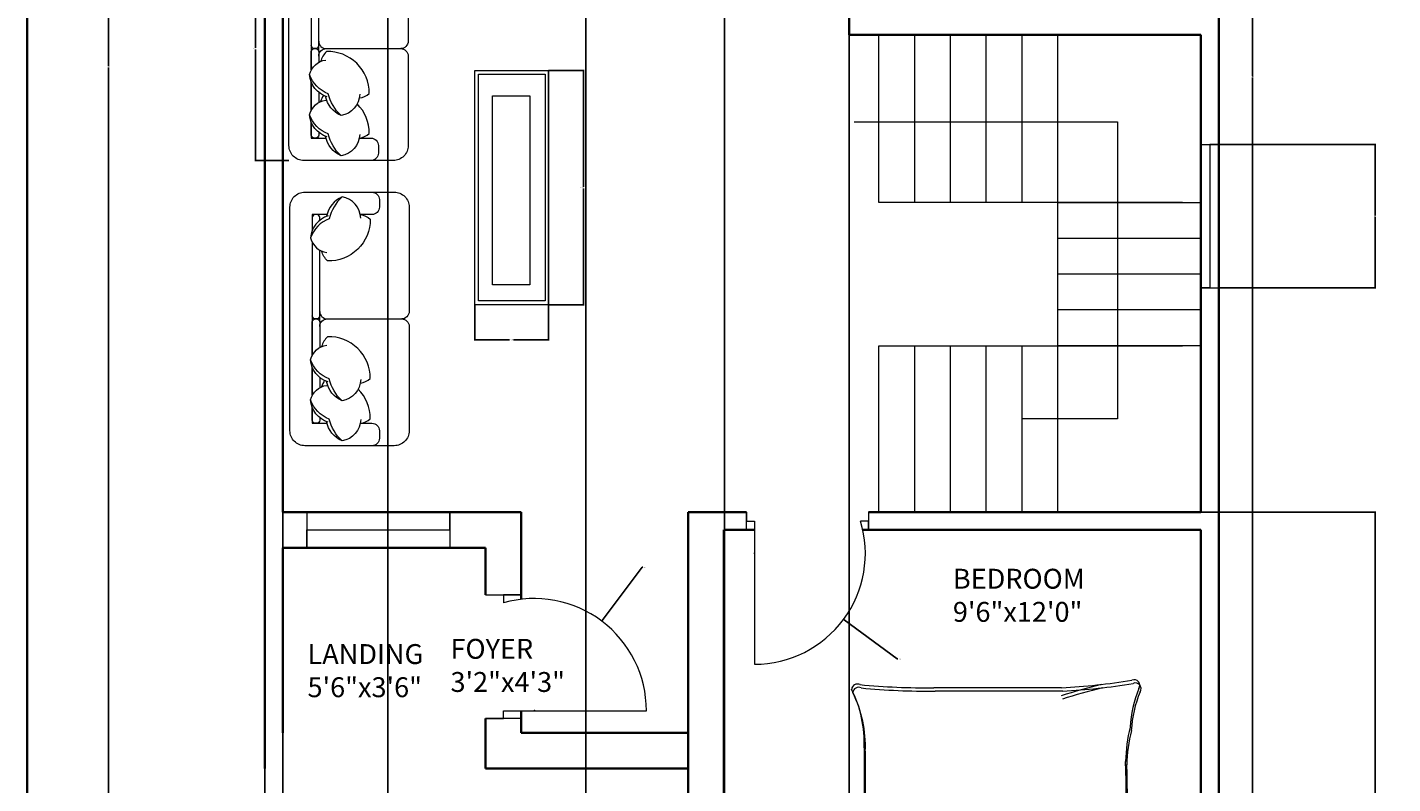
# Model space of a CAD drawing. Units: inches. Extents: x 1734 to 2405, y 1500 to 2491.
# Tile 7 of 14: x 1734 to 2078, y 1888 to 2078. Entities that reach past the tile are written whole.
import ezdxf

# ---------------------------------------------------------------- set-up
doc = ezdxf.new("R2010")
doc.units = ezdxf.units.IN
for name, color, linetype, lineweight in [('A-ANNO-DIMS', 2, 'Continuous', 18), ('A-ANNO-TTLB', 7, 'Continuous', 35), ('A-AREA-IDEN', 7, 'Continuous', 18), ('A-DOOR', 3, 'Continuous', 18), ('A-FLOR-STRS', 7, 'Continuous', 18), ('A-FURN', 8, 'Continuous', 13), ('A-GLAZ', 4, 'Continuous', 18), ('A-WALL', 7, 'Continuous', 35), ('C-PROP', 7, 'Continuous', 25)]:
    doc.layers.add(name, color=color, linetype=linetype, lineweight=lineweight)
doc.styles.get("Standard").update_dxf_attribs({"font": 'arial.ttf'})
doc.dimstyles.get("Standard").update_dxf_attribs({"dimtxt": 0.18, "dimasz": 0.18, "dimexe": 0.18, "dimexo": 0.0625, "dimgap": 0.09, "dimtad": 0, "dimtih": 1, "dimtoh": 1, "dimdec": 4, "dimzin": 0, "dimdsep": 46, "dimtxsty": 'Standard', "dimcen": 0.09, "dimadec": 0, "dimazin": 0, "dimtfac": 1, "dimtdec": 4, "dimtofl": 0, "dimtmove": 0, "dimatfit": 3, "dimfxl": 1, "dimtolj": 1, "dimtzin": 0, "dimarcsym": 0})

# ---------------------------------------------------------------- blocks, each defined once
blk = doc.blocks.new('BED-DOUBLE')
for p, q in [((81.88, 67.96), (105.53, 67.96)), ((81.88, 67.96), (105.53, 67.96)), ((82.71, 68.26), (106.37, 68.26)), ((82.71, 68.26), (106.37, 68.26)), ((83.83, 60.38), (82.88, 67.03)), ((82.88, 67.03), (87.04, 66.28)), ((83.83, 60.38), (82.88, 67.03)), ((82.88, 67.03), (87.04, 66.28)), ((84.66, 60.68), (83.72, 67.33)), ((83.72, 67.33), (87.87, 66.58)), ((84.66, 60.68), (83.72, 67.33)), ((83.72, 67.33), (87.87, 66.58)), ((87.04, 66.28), (89.12, 66.66)), ((87.04, 66.28), (89.12, 66.66)), ((87.87, 66.58), (89.95, 66.95)), ((87.87, 66.58), (89.95, 66.95)), ((89.12, 66.66), (93.84, 65.9)), ((89.12, 66.66), (93.84, 65.9)), ((89.95, 66.95), (94.67, 66.2)), ((89.95, 66.95), (94.67, 66.2)), ((93.65, 67.22), (92.33, 66.47)), ((93.65, 67.22), (92.33, 66.47)), ((94.48, 67.52), (93.16, 66.77)), ((94.48, 67.52), (93.16, 66.77)), ((97.05, 66.66), (93.65, 67.22)), ((97.05, 66.66), (93.65, 67.22)), ((93.84, 65.9), (97.42, 64.58)), ((93.84, 65.9), (97.42, 64.58)), ((97.88, 66.95), (94.48, 67.52)), ((97.88, 66.95), (94.48, 67.52)), ((94.67, 66.2), (98.26, 64.88)), ((94.67, 66.2), (98.26, 64.88)), ((101.2, 67.41), (97.05, 66.66)), ((101.2, 67.41), (97.05, 66.66)), ((102.04, 67.71), (97.88, 66.95)), ((102.04, 67.71), (97.88, 66.95)), ((101.17, 67.41), (101.6, 61.81)), ((101.17, 67.41), (101.6, 61.82)), ((102.01, 67.7), (102.44, 62.11)), ((102.01, 67.7), (102.44, 62.11)), ((103.53, 67.96), (103.53, 5.54)), ((103.53, 67.96), (103.53, 5.54)), ((104.36, 68.26), (104.36, 5.84)), ((104.36, 68.26), (104.36, 5.84)), ((106.37, 5.54), (106.37, 67.96)), ((85.12, 64.16), (84.25, 58.9)), ((85.12, 64.16), (84.25, 58.9)), ((85.96, 64.46), (85.09, 59.2)), ((85.96, 64.46), (85.09, 59.2)), ((102.41, 61.98), (102.04, 56.98)), ((102.41, 61.98), (102.04, 56.98)), ((102.44, 62.11), (102.41, 61.98)), ((102.44, 62.11), (102.41, 61.98)), ((84.25, 58.9), (83.69, 49.74)), ((84.25, 58.9), (83.69, 49.74)), ((84.25, 58.9), (83.83, 60.38)), ((84.25, 58.9), (83.83, 60.38)), ((85.09, 59.2), (84.52, 50.04)), ((85.09, 59.2), (84.52, 50.04)), ((85.09, 59.2), (84.66, 60.68)), ((85.09, 59.2), (84.66, 60.68)), ((101.58, 61.68), (101.2, 56.68)), ((101.58, 61.68), (101.2, 56.68)), ((101.6, 61.82), (101.58, 61.68)), ((101.6, 61.81), (101.58, 61.68)), ((101.2, 56.68), (99.88, 49.51)), ((101.2, 56.68), (99.88, 49.51)), ((102.04, 56.98), (100.71, 49.81)), ((102.04, 56.98), (100.71, 49.81)), ((2.04, 52.82), (2.04, 20.68)), ((2.04, 52.82), (2.04, 20.68)), ((2.87, 53.12), (2.87, 20.98)), ((2.87, 53.12), (2.87, 20.98)), ((100.64, 53.1), (101.58, 50.45)), ((100.64, 53.1), (101.58, 50.45)), ((101.47, 53.4), (102.41, 50.75)), ((101.47, 53.39), (102.41, 50.75)), ((83.69, 49.74), (84.42, 47.18)), ((83.69, 49.74), (84.42, 47.18)), ((84.52, 50.04), (85.25, 47.48)), ((84.52, 50.04), (85.25, 47.48)), ((101.58, 50.45), (102.52, 46.68)), ((101.58, 50.45), (102.52, 46.68)), ((102.41, 50.75), (103.36, 46.98)), ((102.41, 50.75), (103.36, 46.98)), ((84.42, 47.18), (83.89, 40.48)), ((84.42, 47.18), (83.89, 40.48)), ((84.29, 41.02), (85.72, 45.13)), ((84.29, 41.02), (85.72, 45.12)), ((85.25, 47.48), (84.72, 40.78)), ((85.25, 47.48), (84.72, 40.78)), ((85.13, 41.32), (86.55, 45.42)), ((85.13, 41.32), (86.55, 45.42)), ((102.52, 46.26), (102.33, 40.45)), ((102.52, 46.26), (102.33, 40.45)), ((102.52, 46.68), (102.52, 46.26)), ((102.52, 46.68), (102.52, 46.26)), ((103.36, 46.56), (103.17, 40.75)), ((103.36, 46.56), (103.17, 40.75)), ((103.36, 46.98), (103.36, 46.56)), ((103.36, 46.98), (103.36, 46.56)), ((85.13, 38.11), (85.13, 41.32)), ((85.13, 38.11), (85.13, 41.32)), ((84.29, 37.81), (84.29, 41.02)), ((84.29, 37.81), (84.29, 41.02)), ((87.79, 37.81), (84.29, 37.81)), ((87.79, 37.81), (84.29, 37.81)), ((88.63, 38.11), (85.13, 38.11)), ((88.63, 38.11), (85.13, 38.11)), ((90.25, 37.05), (87.79, 37.81)), ((90.25, 37.05), (87.79, 37.81)), ((91.08, 37.35), (88.63, 38.11)), ((91.08, 37.35), (88.63, 38.11)), ((96.1, 37.81), (91.95, 37.05)), ((96.1, 37.81), (91.95, 37.05)), ((96.94, 38.11), (92.78, 37.35)), ((96.94, 38.11), (92.78, 37.35)), ((103.09, 38.56), (96.1, 37.81)), ((103.09, 38.56), (96.1, 37.81)), ((103.92, 38.86), (96.94, 38.11)), ((103.92, 38.86), (96.94, 38.11)), ((102.33, 40.45), (103.09, 38.56)), ((102.33, 40.45), (103.09, 38.56)), ((103.17, 40.75), (103.92, 38.86)), ((103.17, 40.75), (103.92, 38.86)), ((86.97, 35.76), (83.47, 35.54)), ((86.97, 35.76), (83.47, 35.54)), ((83.47, 35.54), (83.67, 32.34)), ((83.47, 35.54), (83.67, 32.34)), ((87.8, 36.06), (84.3, 35.84)), ((87.8, 36.06), (84.3, 35.84)), ((84.3, 35.84), (84.51, 32.63)), ((84.3, 35.84), (84.51, 32.64)), ((89.37, 36.67), (86.97, 35.76)), ((89.37, 36.67), (86.97, 35.76)), ((90.2, 36.96), (87.8, 36.06)), ((90.2, 36.96), (87.8, 36.06)), ((91.06, 36.77), (89.37, 36.67)), ((91.06, 36.77), (89.37, 36.67)), ((91.9, 37.07), (90.2, 36.96)), ((91.9, 37.07), (90.2, 36.96)), ((91.95, 37.05), (90.25, 37.05)), ((91.95, 37.05), (90.25, 37.05)), ((95.26, 36.28), (91.06, 36.77)), ((95.26, 36.28), (91.06, 36.77)), ((92.78, 37.35), (91.08, 37.35)), ((92.78, 37.35), (91.08, 37.35)), ((96.09, 36.57), (91.9, 37.07)), ((96.09, 36.58), (91.9, 37.07)), ((102.28, 35.96), (95.26, 36.28)), ((102.28, 35.96), (95.26, 36.28)), ((103.11, 36.26), (96.09, 36.58)), ((103.11, 36.26), (96.09, 36.57)), ((101.64, 34.03), (102.28, 35.96)), ((101.64, 34.03), (102.28, 35.96)), ((102.48, 34.33), (103.11, 36.26)), ((102.48, 34.33), (103.11, 36.26)), ((82.83, 32.98), (74.35, 27.51)), ((82.83, 32.98), (74.35, 27.51)), ((83.66, 33.28), (75.18, 27.8)), ((83.66, 33.28), (75.18, 27.8)), ((83.67, 32.34), (85.35, 28.33)), ((83.67, 32.34), (85.35, 28.33)), ((84.51, 32.64), (86.18, 28.63)), ((84.51, 32.63), (86.18, 28.62)), ((102.19, 28.24), (101.64, 34.03)), ((102.19, 28.24), (101.64, 34.03)), ((103.03, 28.54), (102.48, 34.33)), ((103.03, 28.54), (102.48, 34.33)), ((74.35, 27.51), (68.49, 25.28)), ((74.35, 27.51), (68.49, 25.28)), ((75.18, 27.8), (69.32, 25.58)), ((75.18, 27.8), (69.32, 25.58)), ((79, 19.42), (82.83, 30.31)), ((79, 19.41), (82.83, 30.3)), ((79.83, 19.71), (83.66, 30.6)), ((79.83, 19.71), (83.66, 30.6)), ((85.12, 29.97), (84.25, 24.7)), ((85.12, 29.97), (84.25, 24.7)), ((85.96, 30.27), (85.09, 25)), ((85.96, 30.27), (85.09, 25)), ((101.51, 24), (102.22, 27.83)), ((101.51, 24), (102.22, 27.83)), ((102.22, 27.83), (102.19, 28.24)), ((102.22, 27.83), (102.19, 28.24)), ((102.35, 24.3), (103.05, 28.12)), ((102.35, 24.3), (103.05, 28.12)), ((103.05, 28.12), (103.03, 28.54)), ((103.05, 28.12), (103.03, 28.54)), ((68.49, 25.28), (65.86, 24.88)), ((68.49, 25.28), (65.86, 24.88)), ((65.86, 24.88), (66.67, 21.64)), ((65.86, 24.88), (66.67, 21.64)), ((69.32, 25.58), (66.69, 25.17)), ((69.32, 25.58), (66.69, 25.17)), ((66.69, 25.17), (67.5, 21.94)), ((66.69, 25.17), (67.5, 21.94)), ((84.25, 24.7), (83.69, 15.55)), ((84.25, 24.7), (83.69, 15.55)), ((85.09, 25), (84.52, 15.84)), ((85.09, 25), (84.52, 15.85)), ((101.52, 17.76), (99.76, 24.83)), ((101.52, 17.76), (99.76, 24.83)), ((102.36, 18.05), (100.59, 25.13)), ((102.36, 18.05), (100.59, 25.13)), ((101.57, 21.6), (102.35, 24.3)), ((101.57, 21.6), (102.35, 24.3)), ((66.67, 21.64), (67.88, 19.01)), ((66.67, 21.64), (67.88, 19.01)), ((67.5, 21.94), (68.72, 19.31)), ((67.5, 21.94), (68.72, 19.31)), ((100.73, 21.3), (101.51, 24)), ((100.73, 21.3), (101.51, 24)), ((67.88, 19.01), (68.49, 14.56)), ((67.88, 19.01), (68.49, 14.56)), ((68.72, 19.31), (69.32, 14.86)), ((68.72, 19.31), (69.32, 14.86)), ((76.37, 12.13), (79, 19.42)), ((76.37, 12.13), (79, 19.41)), ((77.21, 12.43), (79.83, 19.71)), ((77.21, 12.43), (79.83, 19.71)), ((102.21, 12.8), (101.52, 17.76)), ((102.21, 12.8), (101.52, 17.76)), ((103.05, 13.09), (102.36, 18.05)), ((103.05, 13.09), (102.36, 18.05)), ((68.49, 14.56), (68.89, 9.5)), ((68.49, 14.56), (68.89, 9.5)), ((69.32, 14.86), (69.73, 9.8)), ((69.32, 14.86), (69.73, 9.8)), ((83.69, 15.55), (84.42, 12.99)), ((83.69, 15.55), (84.42, 12.99)), ((84.52, 15.85), (85.25, 13.28)), ((84.52, 15.84), (85.25, 13.28)), ((102.19, 7.05), (102.32, 14.11)), ((102.19, 7.05), (102.32, 14.11)), ((102.32, 14.11), (102.21, 12.8)), ((102.32, 14.11), (102.21, 12.8)), ((103.03, 7.35), (103.15, 14.4)), ((103.03, 7.35), (103.15, 14.4)), ((103.15, 14.4), (103.05, 13.09)), ((103.15, 14.4), (103.05, 13.09)), ((73.54, 8.29), (76.37, 12.13)), ((73.54, 8.29), (76.37, 12.13)), ((74.38, 8.59), (77.21, 12.43)), ((74.38, 8.59), (77.21, 12.43)), ((84.42, 12.99), (83.89, 6.28)), ((84.42, 12.99), (83.89, 6.28)), ((85.25, 13.28), (84.72, 6.58)), ((85.25, 13.28), (84.72, 6.58)), ((68.89, 9.5), (68.49, 5.46)), ((68.89, 9.5), (68.49, 5.46)), ((69.3, 3.45), (73.54, 8.29)), ((69.3, 3.45), (73.54, 8.29)), ((69.73, 9.8), (69.32, 5.76)), ((69.73, 9.8), (69.32, 5.76)), ((70.13, 3.75), (74.38, 8.59)), ((70.13, 3.75), (74.38, 8.59)), ((83.89, 6.28), (87.99, 7.3)), ((83.89, 6.28), (87.99, 7.3)), ((84.72, 6.58), (88.82, 7.6)), ((84.72, 6.58), (88.82, 7.59)), ((87.99, 7.3), (90.08, 7.05)), ((87.99, 7.3), (90.08, 7.05)), ((88.82, 7.6), (90.92, 7.35)), ((88.82, 7.59), (90.92, 7.35)), ((90.08, 7.05), (94.75, 8.1)), ((90.08, 7.05), (94.75, 8.1)), ((90.92, 7.35), (95.58, 8.4)), ((90.92, 7.35), (95.58, 8.4)), ((94.64, 6.77), (93.28, 7.44)), ((94.64, 6.77), (93.28, 7.44)), ((95.48, 7.07), (94.11, 7.74)), ((95.48, 7.07), (94.11, 7.74)), ((98, 7.54), (94.64, 6.77)), ((98, 7.54), (94.64, 6.77)), ((94.75, 8.1), (98.25, 9.64)), ((94.75, 8.1), (98.25, 9.64)), ((98.83, 7.84), (95.48, 7.07)), ((98.83, 7.84), (95.48, 7.07)), ((95.58, 8.4), (99.08, 9.94)), ((95.58, 8.4), (99.08, 9.94)), ((102.19, 7.05), (98, 7.54)), ((102.19, 7.05), (98, 7.54)), ((103.03, 7.35), (98.83, 7.84)), ((103.03, 7.35), (98.83, 7.84)), ((67.02, 3.35), (69.3, 3.45, 5.06)), ((67.02, 3.35), (69.3, 3.45, 5.06)), ((67.85, 3.65), (70.13, 3.75, 5.06)), ((67.85, 3.65), (70.13, 3.75, 5.06)), ((68.49, 5.46), (69.3, 3.45)), ((68.49, 5.46), (69.3, 3.45)), ((69.32, 5.76), (70.13, 3.75)), ((69.32, 5.76), (70.13, 3.75)), ((105.53, 5.54), (70.78, 5.54)), ((105.53, 5.54), (70.78, 5.54)), ((106.37, 5.84), (71.61, 5.84)), ((106.37, 5.84), (71.61, 5.84)), ((106.37, 5.54), (105.53, 5.54))]:
    blk.add_line(p, q)
for centre, radius, start, end in [((1.42, 71.08), 1.42, 56.1736, 203.4781), ((1.42, 71.08), 1.42, 56.1736, 203.4781), ((2.25, 71.38), 1.42, 56.1736, 203.4781), ((2.25, 71.38), 1.42, 56.1736, 203.4781), ((13.75, 100.79), 30.77, 247.9751, 266.652), ((13.75, 100.79), 30.77, 247.9751, 266.652), ((14.58, 101.08), 30.77, 247.9751, 266.652), ((14.58, 101.08), 30.77, 247.9751, 266.652), ((-156.77, 44.51), 159.02, 2.9958, 9.4091), ((-156.77, 44.51), 159.02, 2.9958, 9.4091), ((-155.93, 44.81), 159.02, 2.9958, 9.4091), ((-155.93, 44.81), 159.02, 2.9958, 9.4091), ((21.27, 107.63), 38.7, 256.0648, 268.9113), ((21.27, 107.63), 38.7, 256.0648, 268.9113), ((22.11, 107.93), 38.7, 256.0648, 268.9113), ((22.11, 107.93), 38.7, 256.0648, 268.9113), ((39.43, -560.7), 629.91, 88.22771, 91.71854), ((39.43, -560.7), 629.91, 88.22771, 91.71854), ((40.26, -560.4), 629.91, 88.22771, 91.71854), ((40.26, -560.4), 629.91, 88.22771, 91.71854), ((64.82, 291.01), 222.17, 268.4762, 271.0082), ((64.82, 291.01), 222.17, 268.4762, 271.0082), ((65.65, 291.31), 222.17, 268.4762, 271.0082), ((65.65, 291.31), 222.17, 268.4762, 271.0082), ((-98.62, 49.31), 168.5, 351.7845, 6.9006), ((-98.62, 49.31), 168.5, 351.7845, 6.9006), ((79.29, -38.73), 108.8, 88.7218, 95.604), ((79.29, -38.73), 108.8, 88.7218, 95.604), ((-97.79, 49.61), 168.5, 351.7845, 6.9006), ((-97.79, 49.61), 168.5, 351.7845, 6.9006), ((80.12, -38.43), 108.8, 88.7218, 95.604), ((80.12, -38.43), 108.8, 88.7218, 95.604), ((-132.23, 44.6), 215.46, 356.0865, 6.7821), ((-132.23, 44.6), 215.46, 356.0865, 6.7821), ((-131.4, 44.9), 215.46, 356.0865, 6.7821), ((-131.4, 44.9), 215.46, 356.0865, 6.7821), ((136.5, 94.99), 139.04, 193.3832, 197.7053), ((136.5, 94.99), 139.04, 193.3832, 197.7053), ((137.34, 95.29), 139.04, 193.3832, 197.7053), ((137.34, 95.29), 139.04, 193.3832, 197.7053), ((65.78, 24.65), 0.241, 70.2464, 181.1377), ((65.78, 24.65), 0.241, 70.2464, 181.1377), ((103.6, 31.81), 38.73, 190.6617, 199.8806), ((103.6, 31.81), 38.73, 190.6617, 199.8806), ((66.61, 24.95), 0.241, 70.2464, 181.1377), ((66.61, 24.95), 0.241, 70.2464, 181.1377), ((104.43, 32.11), 38.73, 190.6617, 199.8806), ((104.43, 32.11), 38.73, 190.6617, 199.8806), ((-171.71, 18.75), 173.75, 354.4998, 0.6351), ((-171.71, 18.75), 173.75, 354.4998, 0.6351), ((-170.87, 19.05), 173.75, 354.4998, 0.6351), ((-170.87, 19.05), 173.75, 354.4998, 0.6351), ((59.73, 15.37), 8.13, 348.6608, 23.7384), ((59.73, 15.37), 8.13, 348.6608, 23.7384), ((60.57, 15.67), 8.13, 348.6608, 23.7384), ((60.57, 15.67), 8.13, 348.6608, 23.7384), ((114.23, 5.46), 47.26, 169.8763, 182.5657), ((114.23, 5.46), 47.26, 169.8763, 182.5657), ((115.06, 5.76), 47.26, 169.8763, 182.5657), ((115.06, 5.76), 47.26, 169.8763, 182.5657), ((16.69, -26.67), 30.12, 87.4714, 116.4681), ((16.69, -26.67), 30.12, 87.4714, 116.4681), ((17.79, 5961.38), 5957.95, 270.002168, 270.286887), ((17.79, 5961.38), 5957.95, 270.002168, 270.286887), ((58.1, -165.55), 169.13, 86.9791, 93.8365), ((58.1, -165.55), 169.13, 86.9791, 93.8365), ((58.94, -165.25), 169.13, 86.9791, 93.8365), ((58.94, -165.25), 169.13, 86.9791, 93.8365), ((2.53, 1.44), 1.44, 152.6588, 266.02), ((2.53, 1.44), 1.44, 152.6588, 266.02), ((3.36, 1.73), 1.44, 152.6588, 266.02), ((3.36, 1.74), 1.44, 152.6588, 266.02), ((15.85, -26.97), 30.12, 87.4714, 116.4681), ((15.85, -26.97), 30.12, 87.4714, 116.4681), ((16.96, 5961.08), 5957.95, 270.002168, 270.286887), ((16.96, 5961.08), 5957.95, 270.002168, 270.286887)]:
    blk.add_arc(centre, radius, start, end)
blk = doc.blocks.new('SOFA-COMPACT')
at = {"ltscale": 0.03}
blk.add_lwpolyline([(29.99, 29.99, -0.414214), (28.12, 28.12, -0.414214), (29.99, 26.24), (29.99, 3.75, -0.414214), (26.24, 0), (3.75, 0, -0.414214), (0, 3.75), (0, 52.49, -0.414214), (3.75, 56.24), (26.24, 56.24, -0.414214), (29.99, 52.49), (29.99, 29.99, -0.414214), (28.12, 28.12, -0.414214), (29.99, 26.24)], format="xyb", dxfattribs=at)
for points in [[(13.1, 55.04, 0.14773), (9.88, 49.56, 0.213343), (5.16, 44.73, 0.178662)], [(17.83, 49.67, 0.356772), (13.1, 55.04, 0.249542), (9.21, 50.18, -9.61688)], [(20.62, 56.24, -0.414214), (22.49, 54.36), (22.49, 52.49, -0.414214), (20.62, 50.61), (17.72, 50.61)], [(9.63, 50.32, 0.306663), (5.16, 44.73, 0.30633), (9.24, 41.08, -0.872847)], [(7.5, 49.18), (7.5, 49.86, 0.414214), (6.75, 50.61), (6.37, 50.61, 0.414214), (5.62, 49.86)], [(5.62, 49.86), (5.62, 46.67, 0.414214)], [(17.71, 50.62, -0.165541), (20.19, 49.46, -0.425989), (9.45, 38.93, -0.121523), (7.97, 41.43, 7.115464)], [(5.62, 43.55), (5.62, 28.87, 0.414214), (6.37, 28.12), (6.75, 28.12, 0.414214), (7.5, 28.87), (7.5, 41.66, 0.414214)], [(5.62, 22.78), (5.62, 27.37, -0.414214), (6.37, 28.12), (6.75, 28.12, -0.414214), (7.5, 27.37), (7.5, 24.67, -0.414214)], [(7.5, 29.99, 0.414214), (9.37, 28.12)], [(7.5, 29.99, 0.414214), (9.37, 28.12), (28.12, 28.12, 0.414214)], [(7.5, 26.24, -0.414214), (9.37, 28.12)], [(7.5, 26.24, -0.414214), (9.37, 28.12), (28.12, 28.12, -0.414214)], [(9.63, 16.01, -0.306663), (5.16, 21.6, -0.30633), (9.24, 25.26, 0.872847)], [(17.71, 15.72, 0.165541), (20.19, 16.88, 0.425989), (9.45, 27.4, 0.121523), (7.97, 24.91, -7.115464)], [(13.1, 11.29, -0.14773), (9.88, 16.77, -0.213343), (5.16, 21.6, -0.178662)], [(5.62, 12.69), (5.62, 19.67, -0.414214)], [(9.63, 5.91, -0.306663), (5.16, 11.51, -0.30633), (9.24, 15.16, 0.872847)], [(7.5, 17.15), (7.5, 14.57, -0.414214)], [(8.71, 16.38, 0.071865), (7.97, 14.81, -7.115464)], [(17.83, 16.66, -0.356772), (13.1, 11.29, -0.249542), (9.21, 16.16, 9.61688)], [(17.71, 5.62, 0.165541), (20.19, 6.78, 0.200231), (17.17, 14.22, 0.121523)], [(13.1, 1.19, -0.14773), (9.88, 6.67, -0.213343), (5.16, 11.51, -0.178662)], [(5.62, 6.37), (5.62, 9.57, -0.414214)], [(5.62, 9.57), (5.62, 5.62), (9.31, 5.62, -0.414214)], [(7.5, 7.05), (7.5, 6.37, -0.414214), (6.75, 5.62), (6.37, 5.62, -0.414214), (5.62, 6.37)], [(17.83, 6.56, -0.356772), (13.1, 1.19, -0.249542), (9.21, 6.06, 9.61688)], [(17.72, 5.62), (20.62, 5.62, -0.414214), (22.49, 3.75), (22.49, 1.87, -0.414214), (20.62, 0)]]:
    blk.add_lwpolyline(points, format="xyb")
for points in [[(9.31, 50.61), (5.62, 50.61), (5.62, 46.67)], [(5.62, 43.55), (5.62, 22.78)], [(5.62, 19.67), (5.62, 12.69)]]:
    blk.add_lwpolyline(points)
blk.add_lwpolyline([(5.62, 28.87), (5.62, 27.37, -0.414214), (6.37, 28.12), (6.75, 28.12, -0.414214), (7.5, 27.37), (7.5, 28.87, -0.414214), (6.75, 28.12), (6.37, 28.12, -0.414214)], format="xyb", close=True)
blk = doc.blocks.new('SOFA-LONG')
at = {"ltscale": 0.03}
blk.add_lwpolyline([(29.99, 33.74, -0.414214), (28.12, 31.87, -0.414214), (29.99, 29.99), (29.99, 3.75, -0.414214), (26.24, 0), (3.75, 0, -0.414214), (0, 3.75), (0, 59.98, -0.414214), (3.75, 63.73), (26.24, 63.73, -0.414214), (29.99, 59.98), (29.99, 33.74, -0.414214), (28.12, 31.87, -0.414214), (29.99, 29.99)], format="xyb", dxfattribs=at)
for points in [[(13.1, 62.54, 0.14773), (9.88, 57.06, 0.213343), (5.16, 52.23, 0.178662)], [(17.83, 57.17, 0.356772), (13.1, 62.54, 0.249542), (9.21, 57.67, -9.61688)], [(20.62, 63.73, -0.414214), (22.49, 61.86), (22.49, 59.98, -0.414214), (20.62, 58.11), (17.71, 58.11)], [(9.63, 57.82, 0.306663), (5.16, 52.23, 0.30633), (9.24, 48.58, -0.872847)], [(7.5, 56.68), (7.5, 57.36, 0.414214), (6.75, 58.11), (6.37, 58.11, 0.414214), (5.62, 57.36)], [(5.62, 57.36), (5.62, 54.17, 0.414214)], [(17.71, 58.11, -0.165541), (20.19, 56.95, -0.425989), (9.45, 46.43, -0.121523), (7.97, 48.93, 7.115464)], [(5.62, 51.05), (5.62, 32.62, 0.414214), (6.37, 31.87), (6.75, 31.87, 0.414214), (7.5, 32.62), (7.5, 49.16, 0.414214)], [(5.62, 22.78), (5.62, 31.12, -0.414214), (6.37, 31.87), (6.75, 31.87, -0.414214), (7.5, 31.12), (7.5, 24.67, -0.414214)], [(7.5, 33.74, 0.414214), (9.37, 31.87)], [(7.5, 33.74, 0.414214), (9.37, 31.87), (28.12, 31.87, 0.414214)], [(7.5, 29.99, -0.414214), (9.37, 31.87)], [(7.5, 29.99, -0.414214), (9.37, 31.87), (28.12, 31.87, -0.414214)], [(9.63, 16.01, -0.306663), (5.16, 21.6, -0.30633), (9.24, 25.26, 0.872847)], [(17.71, 15.72, 0.165541), (20.19, 16.88, 0.425989), (9.45, 27.4, 0.121523), (7.97, 24.91, -7.115464)], [(13.1, 11.29, -0.14773), (9.88, 16.77, -0.213343), (5.16, 21.6, -0.178662)], [(5.62, 12.69), (5.62, 19.67, -0.414214)], [(9.63, 5.92, -0.306663), (5.16, 11.51, -0.30633), (9.24, 15.16, 0.872847)], [(7.5, 17.15), (7.5, 14.57, -0.414214)], [(8.71, 16.38, 0.071865), (7.97, 14.81, -7.115464)], [(17.83, 16.66, -0.356772), (13.1, 11.29, -0.249542), (9.21, 16.16, 9.61688)], [(17.71, 5.62, 0.165541), (20.19, 6.78, 0.200231), (17.17, 14.22, 0.121523)], [(13.1, 1.19, -0.14773), (9.88, 6.67, -0.213343), (5.16, 11.51, -0.178662)], [(5.62, 9.57), (5.62, 5.62), (9.31, 5.62, -0.414214)], [(5.62, 6.37), (5.62, 9.57, -0.414214)], [(7.5, 7.05), (7.5, 6.37, -0.414214), (6.75, 5.62), (6.37, 5.62, -0.414214), (5.62, 6.37)], [(17.83, 6.56, -0.356772), (13.1, 1.19, -0.249542), (9.21, 6.06, 9.61688)], [(17.71, 5.62), (20.62, 5.62, -0.414214), (22.49, 3.75), (22.49, 1.87, -0.414214), (20.62, 0)]]:
    blk.add_lwpolyline(points, format="xyb")
for points in [[(9.31, 58.11), (5.62, 58.11), (5.62, 54.17)], [(5.62, 51.05), (5.62, 22.78)], [(5.62, 19.67), (5.62, 12.69)]]:
    blk.add_lwpolyline(points)
blk.add_lwpolyline([(5.62, 32.62), (5.62, 31.12, -0.414214), (6.37, 31.87), (6.75, 31.87, -0.414214), (7.5, 31.12), (7.5, 32.62, -0.414214), (6.75, 31.87), (6.37, 31.87, -0.414214)], format="xyb", close=True)
blk = doc.blocks.new('TABLE-COFFEE')
for points in [[(0, 58.87), (18.49, 58.87), (18.49, 0), (0, 0)], [(0.91, 57.96), (17.71, 57.96), (17.71, 0.97), (0.91, 0.97)], [(4.43, 52.52), (13.86, 52.52), (13.86, 5), (4.43, 5)]]:
    blk.add_lwpolyline(points, close=True)
blk = doc.blocks.new('*D12')
at = {"layer": 'A-ANNO-DIMS', "color": 0, "lineweight": -2, "transparency": 16777216}
for p, q in [((1799.89, 2100.96), (1791.34, 2100.96)), ((1791.52, 2100.78), (1791.52, 2073.03)), ((1791.52, 2044.91), (1791.52, 2072.66)), ((1799.89, 2044.73), (1791.34, 2044.73))]:
    blk.add_line(p, q, dxfattribs=at)
at = {"layer": 'A-ANNO-DIMS', "color": 0, "transparency": 16777216}
for points in [[(1791.49, 2100.78), (1791.55, 2100.78), (1791.52, 2100.96)], [(1791.49, 2044.91), (1791.55, 2044.91), (1791.52, 2044.73)]]:
    blk.add_solid(points, dxfattribs=at)
at = {"layer": 'Defpoints', "color": 0, "transparency": 16777216}
for p in [(1791.52, 2100.96), (1799.96, 2100.96), (1799.96, 2044.73)]:
    blk.add_point(p, dxfattribs=at)
at = {"layer": 'A-ANNO-DIMS', "color": 0, "transparency": 16777216, "insert": (1791.52, 2072.84), "char_height": 0.18, "attachment_point": 5}
blk.add_mtext('\\A1;SOFA 56 TYP.', dxfattribs=at)
blk = doc.blocks.new('*D16')
at = {"layer": 'A-ANNO-DIMS', "color": 0, "lineweight": -2, "transparency": 16777216}
for p, q in [((1865.28, 2067.33), (1874.23, 2067.33)), ((1874.05, 2067.15), (1874.05, 2038.07)), ((1874.05, 2008.64), (1874.05, 2037.71)), ((1865.28, 2008.46), (1874.23, 2008.46))]:
    blk.add_line(p, q, dxfattribs=at)
at = {"layer": 'A-ANNO-DIMS', "color": 0, "transparency": 16777216}
for points in [[(1874.02, 2067.15), (1874.08, 2067.15), (1874.05, 2067.33)], [(1874.02, 2008.64), (1874.08, 2008.64), (1874.05, 2008.46)]]:
    blk.add_solid(points, dxfattribs=at)
at = {"layer": 'Defpoints', "color": 0, "transparency": 16777216}
for p in [(1865.22, 2067.33), (1874.05, 2067.33), (1865.22, 2008.46)]:
    blk.add_point(p, dxfattribs=at)
at = {"layer": 'A-ANNO-DIMS', "color": 0, "transparency": 16777216, "insert": (1874.05, 2037.89), "char_height": 0.18, "attachment_point": 5}
blk.add_mtext('\\A1;TABLE 59 TYP.', dxfattribs=at)
blk = doc.blocks.new('*D17')
at = {"layer": 'A-ANNO-DIMS', "color": 0, "lineweight": -2, "transparency": 16777216}
for p, q in [((1846.73, 2008.39), (1846.73, 1999.44)), ((1865.22, 2008.39), (1865.22, 1999.44)), ((1846.91, 1999.62), (1855.45, 1999.62)), ((1865.04, 1999.62), (1856.49, 1999.62))]:
    blk.add_line(p, q, dxfattribs=at)
at = {"layer": 'A-ANNO-DIMS', "color": 0, "transparency": 16777216}
for points in [[(1846.91, 1999.65), (1846.91, 1999.59), (1846.73, 1999.62)], [(1865.04, 1999.65), (1865.04, 1999.59), (1865.22, 1999.62)]]:
    blk.add_solid(points, dxfattribs=at)
at = {"layer": 'Defpoints', "color": 0, "transparency": 16777216}
for p in [(1846.73, 2008.46), (1865.22, 2008.46), (1865.22, 1999.62)]:
    blk.add_point(p, dxfattribs=at)
at = {"layer": 'A-ANNO-DIMS', "color": 0, "transparency": 16777216, "insert": (1855.97, 1999.62), "char_height": 0.18, "attachment_point": 5}
blk.add_mtext('\\A1;18 TYP.', dxfattribs=at)
blk = doc.blocks.new('*D23')
at = {"layer": 'A-ANNO-DIMS', "color": 0, "lineweight": -2, "transparency": 16777216}
for p, q in [((1793.83, 2425.82), (1754.36, 2425.82)), ((1754.54, 2425.64), (1754.54, 2068.48)), ((1754.54, 1710.95), (1754.54, 2068.11)), ((1793.83, 1710.77), (1754.36, 1710.77))]:
    blk.add_line(p, q, dxfattribs=at)
at = {"layer": 'A-ANNO-DIMS', "color": 0, "transparency": 16777216}
for points in [[(1754.51, 2425.64), (1754.57, 2425.64), (1754.54, 2425.82)], [(1754.51, 1710.95), (1754.57, 1710.95), (1754.54, 1710.77)]]:
    blk.add_solid(points, dxfattribs=at)
at = {"layer": 'Defpoints', "color": 0, "transparency": 16777216}
for p in [(1754.54, 2425.82), (1793.89, 2425.82), (1793.89, 1710.77)]:
    blk.add_point(p, dxfattribs=at)
at = {"layer": 'A-ANNO-DIMS', "color": 0, "transparency": 16777216, "insert": (1754.54, 2068.3), "char_height": 0.18, "attachment_point": 5}
blk.add_mtext('\\A1;715', dxfattribs=at)
blk = doc.blocks.new('*D27')
at = {"layer": 'A-ANNO-DIMS', "color": 0, "lineweight": -2, "transparency": 16777216}
for p, q in [((2029.46, 1956.32), (2073.42, 1956.32)), ((2073.24, 1956.14), (2073.24, 1877.76)), ((2073.24, 1799), (2073.24, 1877.39)), ((2033.96, 1798.82), (2073.42, 1798.82))]:
    blk.add_line(p, q, dxfattribs=at)
at = {"layer": 'A-ANNO-DIMS', "color": 0, "transparency": 16777216}
for points in [[(2073.21, 1956.14), (2073.27, 1956.14), (2073.24, 1956.32)], [(2073.21, 1799), (2073.27, 1799), (2073.24, 1798.82)]]:
    blk.add_solid(points, dxfattribs=at)
at = {"layer": 'Defpoints', "color": 0, "transparency": 16777216}
for p in [(2029.39, 1956.32), (2073.24, 1956.32), (2033.89, 1798.82)]:
    blk.add_point(p, dxfattribs=at)
at = {"layer": 'A-ANNO-DIMS', "color": 0, "transparency": 16777216, "insert": (2073.24, 1877.57), "char_height": 0.18, "attachment_point": 5}
blk.add_mtext('\\A1;157.5', dxfattribs=at)
blk = doc.blocks.new('*D28')
at = {"layer": 'A-ANNO-DIMS', "color": 0, "lineweight": -2, "transparency": 16777216}
for p, q in [((2033.96, 2048.73), (2073.42, 2048.73)), ((2073.24, 2048.55), (2073.24, 2030.92)), ((2073.24, 2012.91), (2073.24, 2030.55)), ((2033.96, 2012.73), (2073.42, 2012.73))]:
    blk.add_line(p, q, dxfattribs=at)
at = {"layer": 'A-ANNO-DIMS', "color": 0, "transparency": 16777216}
for points in [[(2073.21, 2048.55), (2073.27, 2048.55), (2073.24, 2048.73)], [(2073.21, 2012.91), (2073.27, 2012.91), (2073.24, 2012.73)]]:
    blk.add_solid(points, dxfattribs=at)
at = {"layer": 'Defpoints', "color": 0, "transparency": 16777216}
for p in [(2033.89, 2048.73), (2073.24, 2048.73), (2033.89, 2012.73)]:
    blk.add_point(p, dxfattribs=at)
at = {"layer": 'A-ANNO-DIMS', "color": 0, "transparency": 16777216, "insert": (2073.24, 2030.73), "char_height": 0.18, "attachment_point": 5}
blk.add_mtext('\\A1;36', dxfattribs=at)
blk = doc.blocks.new('*D32')
at = {"layer": 'A-ANNO-DIMS', "color": 0, "lineweight": -2, "transparency": 16777216}
for p, q in [((1798.39, 2202.26), (1798.39, 1615.47)), ((1824.83, 2202.26), (1824.83, 1615.47)), ((1798.57, 1615.65), (1811.22, 1615.65)), ((1824.65, 1615.65), (1812.01, 1615.65))]:
    blk.add_line(p, q, dxfattribs=at)
at = {"layer": 'A-ANNO-DIMS', "color": 0, "transparency": 16777216}
for points in [[(1798.57, 1615.68), (1798.57, 1615.62), (1798.39, 1615.65)], [(1824.65, 1615.68), (1824.65, 1615.62), (1824.83, 1615.65)]]:
    blk.add_solid(points, dxfattribs=at)
at = {"layer": 'Defpoints', "color": 0, "transparency": 16777216}
for p in [(1798.39, 2202.32), (1824.83, 2202.32), (1824.83, 1615.65)]:
    blk.add_point(p, dxfattribs=at)
at = {"layer": 'A-ANNO-DIMS', "color": 0, "transparency": 16777216, "insert": (1811.61, 1615.65), "char_height": 0.18, "attachment_point": 5}
blk.add_mtext('\\A1;26.44', dxfattribs=at)
blk = doc.blocks.new('*D33')
at = {"layer": 'A-ANNO-DIMS', "color": 0, "lineweight": -2, "transparency": 16777216}
for p, q in [((1824.83, 2202.26), (1824.83, 1615.47)), ((1874.68, 2202.26), (1874.68, 1615.47)), ((1825.01, 1615.65), (1849.36, 1615.65)), ((1874.5, 1615.65), (1850.15, 1615.65))]:
    blk.add_line(p, q, dxfattribs=at)
at = {"layer": 'A-ANNO-DIMS', "color": 0, "transparency": 16777216}
for points in [[(1825.01, 1615.68), (1825.01, 1615.62), (1824.83, 1615.65)], [(1874.5, 1615.68), (1874.5, 1615.62), (1874.68, 1615.65)]]:
    blk.add_solid(points, dxfattribs=at)
at = {"layer": 'Defpoints', "color": 0, "transparency": 16777216}
for p in [(1824.83, 2202.32), (1874.68, 2202.32), (1874.68, 1615.65)]:
    blk.add_point(p, dxfattribs=at)
at = {"layer": 'A-ANNO-DIMS', "color": 0, "transparency": 16777216, "insert": (1849.76, 1615.65), "char_height": 0.18, "attachment_point": 5}
blk.add_mtext('\\A1;49.84', dxfattribs=at)
blk = doc.blocks.new('*D34')
at = {"layer": 'A-ANNO-DIMS', "color": 0, "lineweight": -2, "transparency": 16777216}
for p, q in [((1909.52, 2202.26), (1909.52, 1615.47)), ((1940.89, 2204.68), (1940.89, 1615.47)), ((1909.7, 1615.65), (1924.81, 1615.65)), ((1940.71, 1615.65), (1925.6, 1615.65))]:
    blk.add_line(p, q, dxfattribs=at)
at = {"layer": 'A-ANNO-DIMS', "color": 0, "transparency": 16777216}
for points in [[(1909.7, 1615.68), (1909.7, 1615.62), (1909.52, 1615.65)], [(1940.71, 1615.68), (1940.71, 1615.62), (1940.89, 1615.65)]]:
    blk.add_solid(points, dxfattribs=at)
at = {"layer": 'Defpoints', "color": 0, "transparency": 16777216}
for p in [(1909.52, 2202.32), (1940.89, 2204.75), (1940.89, 1615.65)]:
    blk.add_point(p, dxfattribs=at)
at = {"layer": 'A-ANNO-DIMS', "color": 0, "transparency": 16777216, "insert": (1925.21, 1615.65), "char_height": 0.18, "attachment_point": 5}
blk.add_mtext('\\A1;31.37', dxfattribs=at)
blk = doc.blocks.new('*D36')
at = {"layer": 'A-ANNO-DIMS', "color": 0, "lineweight": -2, "transparency": 16777216}
for p, q in [((2081.68, 2425.82), (2042.21, 2425.82)), ((2042.39, 2425.64), (2042.39, 2065.96)), ((2042.39, 1705.92), (2042.39, 2065.6)), ((2081.68, 1705.74), (2042.21, 1705.74))]:
    blk.add_line(p, q, dxfattribs=at)
at = {"layer": 'A-ANNO-DIMS', "color": 0, "transparency": 16777216}
for points in [[(2042.36, 2425.64), (2042.42, 2425.64), (2042.39, 2425.82)], [(2042.36, 1705.92), (2042.42, 1705.92), (2042.39, 1705.74)]]:
    blk.add_solid(points, dxfattribs=at)
at = {"layer": 'Defpoints', "color": 0, "transparency": 16777216}
for p in [(2042.39, 2425.82), (2081.74, 2425.82), (2081.74, 1705.74)]:
    blk.add_point(p, dxfattribs=at)
at = {"layer": 'A-ANNO-DIMS', "color": 0, "transparency": 16777216, "insert": (2042.39, 2065.78), "char_height": 0.18, "attachment_point": 5}
blk.add_mtext('\\A1;720.1', dxfattribs=at)
blk = doc.blocks.new('*D45')
at = {"layer": 'A-ANNO-DIMS', "color": 0, "lineweight": -2, "transparency": 16777216}
for p, q in [((1888.83, 1942.44), (1878.76, 1929.07)), ((1889.01, 1942.44), (1888.83, 1942.44)), ((1861.61, 1906.4), (1861.79, 1906.4)), ((1861.7, 1906.31), (1861.7, 1906.49))]:
    blk.add_line(p, q, dxfattribs=at)
at = {"layer": 'A-ANNO-DIMS', "color": 0, "transparency": 16777216}
blk.add_solid([(1878.74, 1929.09), (1878.79, 1929.05), (1878.65, 1928.92)], dxfattribs=at)
at = {"layer": 'Defpoints', "color": 0, "transparency": 16777216}
for p in [(1878.65, 1928.92), (1861.7, 1906.4)]:
    blk.add_point(p, dxfattribs=at)
at = {"layer": 'A-ANNO-DIMS', "color": 0, "transparency": 16777216, "insert": (1889.42, 1942.44), "char_height": 0.18, "attachment_point": 5}
blk.add_mtext('\\A1;R28.2', dxfattribs=at)
blk = doc.blocks.new('*D46')
at = {"layer": 'A-ANNO-DIMS', "color": 0, "lineweight": -2, "transparency": 16777216}
for p, q in [((1917.01, 1945.95), (1917.19, 1945.95)), ((1917.1, 1945.86), (1917.1, 1946.04)), ((1952.94, 1919.4), (1939.64, 1929.25)), ((1953.12, 1919.4), (1952.94, 1919.4))]:
    blk.add_line(p, q, dxfattribs=at)
at = {"layer": 'A-ANNO-DIMS', "color": 0, "transparency": 16777216}
blk.add_solid([(1939.66, 1929.27), (1939.62, 1929.23), (1939.5, 1929.36)], dxfattribs=at)
at = {"layer": 'Defpoints', "color": 0, "transparency": 16777216}
for p in [(1917.1, 1945.95), (1939.5, 1929.36)]:
    blk.add_point(p, dxfattribs=at)
at = {"layer": 'A-ANNO-DIMS', "color": 0, "transparency": 16777216, "insert": (1953.67, 1919.4), "char_height": 0.18, "attachment_point": 5}
blk.add_mtext('\\A1;R27.875', dxfattribs=at)

msp = doc.modelspace()

# ---------------------------------------------------------------- linework, layer by layer
at = {"layer": 'A-ANNO-TTLB'}
msp.add_lwpolyline([(1734.1307, 2491.1293), (2404.5589, 2491.1293), (2404.5589, 1500.293), (1734.1307, 1500.293)], close=True, dxfattribs=at)
at = {"layer": 'A-DOOR'}
for p, q in [((1915.0984, 1951.8246), (1915.0984, 1956.3246)), ((1915.0984, 1956.3246), (1915.0984, 1954.0746)), ((1945.7636, 1956.3246), (1945.7636, 1951.8246)), ((1915.0984, 1954.0746), (1917.0984, 1954.0746)), ((1917.0984, 1954.0746), (1917.0984, 1918.0746)), ((1945.7636, 1954.0746), (1943.7636, 1954.0746)), ((1945.7636, 1951.8246), (1945.7636, 1954.0746)), ((1849.3942, 1935.4933), (1858.3942, 1935.4933)), ((1858.3942, 1935.4933), (1853.8942, 1935.4933)), ((1853.8942, 1935.4933), (1853.8942, 1933.4933)), ((1858.3942, 1904.3955), (1849.3942, 1904.3955)), ((1849.3942, 1904.3955), (1853.8942, 1904.3955)), ((1853.8942, 1904.3955), (1853.8942, 1906.3955)), ((1853.8942, 1906.3955), (1889.8942, 1906.3955))]:
    msp.add_line(p, q, dxfattribs=at)
for centre, radius, start, end in [((1917.0984, 1945.95), 27.8754, 270, 16.945417), ((1861.6957, 1906.3955), 28.1985, 0, 106.061307)]:
    msp.add_arc(centre, radius, start, end, dxfattribs=at)
at = {"layer": 'A-FLOR-STRS'}
for p, q in [((1948.3942, 2034.1467), (1948.3942, 2076.3246)), ((1957.3942, 2034.1467), (1957.3942, 2076.3246)), ((1966.3942, 2034.1467), (1966.3942, 2076.3246)), ((1975.3942, 2034.1467), (1975.3942, 2076.3246)), ((1984.3942, 2034.1467), (1984.3942, 2076.3246)), ((1993.3942, 2034.1467), (1993.3942, 2076.3246)), ((1942.161, 2054.4364), (2008.3711, 2054.4364)), ((2008.3711, 2054.4364), (2008.3711, 1979.7658)), ((2024.7989, 2034.1467), (1948.3942, 2034.1467)), ((1993.3942, 1998.1467), (1993.3942, 2034.1467)), ((1993.3942, 2034.1467), (2029.3942, 2034.1467)), ((2029.3942, 2025.1467), (1993.3942, 2025.1467)), ((2029.3942, 2016.1467), (1993.3942, 2016.1467)), ((2029.3942, 2007.1467), (1993.3942, 2007.1467)), ((1948.3942, 1956.3246), (1948.3942, 1998.1467)), ((1948.3942, 1998.1467), (2024.7989, 1998.1467)), ((1957.3942, 1956.3246), (1957.3942, 1998.1467)), ((1966.3942, 1956.3246), (1966.3942, 1998.1467)), ((1975.3942, 1956.3246), (1975.3942, 1998.1467)), ((1984.3942, 1956.3246), (1984.3942, 1998.1467)), ((2029.3942, 1998.1467), (1993.3942, 1998.1467)), ((1993.3942, 1956.3246), (1993.3942, 1998.1467)), ((2008.3711, 1979.7658), (1984.3942, 1979.7658))]:
    msp.add_line(p, q, dxfattribs=at)
at = {"layer": 'A-FURN'}
msp.add_lwpolyline([(1846.7266, 2067.3292), (1865.2155, 2067.3292), (1865.2155, 2008.456), (1846.7266, 2008.456)], close=True, dxfattribs=at)
at = {"layer": 'A-GLAZ'}
for p, q in [((2029.3942, 2048.7348), (2029.3942, 2048.7348)), ((2029.3942, 2048.7348), (2033.8942, 2048.7348)), ((2033.8942, 2048.7348), (2031.6442, 2048.7348)), ((2031.6442, 2048.7348), (2031.6442, 2012.7349)), ((2031.6442, 2012.7349), (2029.3942, 2012.7349)), ((2029.3942, 2012.7349), (2033.8942, 2012.7349)), ((1804.4571, 1956.3246), (1804.4571, 1947.3246)), ((1840.4571, 1951.8246), (1840.4571, 1956.3246)), ((1840.4571, 1956.3246), (1840.4571, 1947.3246)), ((1804.4571, 1947.3246), (1804.4571, 1951.8246)), ((1804.4571, 1951.8246), (1840.4571, 1951.8246))]:
    msp.add_line(p, q, dxfattribs=at)
at = {"layer": 'A-WALL'}
for p, q in [((1793.8942, 2425.8246), (1793.8942, 1891.8246)), ((2033.8942, 2425.8246), (2033.8942, 1798.8246)), ((1798.3942, 2202.3246), (1798.3942, 1956.3246)), ((1940.8942, 2085.6314), (1940.8942, 2076.3246)), ((1940.8942, 2076.3246), (2029.3942, 2076.3246)), ((2029.3942, 2076.3246), (2029.3942, 1956.3246)), ((1858.3942, 1956.3246), (1798.3942, 1956.3246)), ((1858.3942, 1947.3246), (1858.3942, 1956.3246)), ((1900.3942, 1956.3246), (1915.0984, 1956.3246)), ((1900.3942, 1956.3246), (1900.3942, 1798.8246)), ((1945.7636, 1956.3246), (2029.3942, 1956.3246)), ((1909.3942, 1951.8246), (1917.0984, 1951.8246)), ((1909.3942, 1951.8246), (1909.3942, 1807.8246)), ((1944.3478, 1951.8246), (2029.3942, 1951.8246)), ((2029.3942, 1951.8246), (2029.3942, 1807.8246)), ((1798.3942, 1947.3246), (1849.3942, 1947.3246)), ((1798.3942, 1947.3246), (1798.3942, 1900.8246)), ((1849.3942, 1935.4933), (1849.3942, 1947.3246)), ((1858.3942, 1947.3246), (1858.3942, 1934.4)), ((1849.3942, 1900.8246), (1849.3942, 1904.3955)), ((1858.3942, 1906.3955), (1858.3942, 1900.8246)), ((1849.3942, 1900.8246), (1849.3942, 1891.8246)), ((1858.3942, 1900.8246), (1900.3942, 1900.8246)), ((1900.3942, 1900.8246), (1862.3942, 1900.8246)), ((1849.3942, 1891.8246), (1900.3942, 1891.8246))]:
    msp.add_line(p, q, dxfattribs=at)
at = {"layer": 'C-PROP'}
for p, q in [((1798.3942, 1900.8246), (1798.3942, 1710.7667)), ((1793.8942, 1891.8246), (1793.8942, 1710.7667))]:
    msp.add_line(p, q, dxfattribs=at)

# ---------------------------------------------------------------- block references
at = {"layer": 'A-FURN'}
for name, p in [('SOFA-COMPACT', (1799.957, 2044.726)), ('TABLE-COFFEE', (1846.727, 2008.456)), ('SOFA-LONG', (1800.209, 1973.025))]:
    msp.add_blockref(name, p, dxfattribs=at)
at = {"layer": 'A-FURN', "rotation": 270}
msp.add_blockref('BED-DOUBLE', (1941.5278, 1914.192), dxfattribs=at)

# ---------------------------------------------------------------- texts
at = {"layer": 'A-AREA-IDEN', "char_height": 5, "attachment_point": 1}
for s, width, insert in [('BEDROOM\\P9\'6"x12\'0"', 80.419691, (1966.9943, 1942.0709)), ('FOYER\\P3\'2"x4\'3"', 32.408377, (1840.6019, 1924.4435)), ('LANDING\\P5\'6"x3\'6"', 63.615528, (1804.629, 1923.1259))]:
    msp.add_mtext_dynamic_manual_height_columns(s, width=width, gutter_width=12.5, heights=[0], dxfattribs=dict(at, insert=insert))

# ---------------------------------------------------------------- dimensions: what is measured, and where the dimension line sits
at = {"layer": 'A-ANNO-DIMS'}
for base, p1, p2, override, picture, middle in [((1754.5442, 2425.8246), (1793.8942, 1710.7667), (1793.8942, 2425.8246), {"dimdec": 0, "dimlfac": 1, "dimrnd": 0, "dimzin": 0, "dimdsep": 46, "dimlunit": 2}, '*D23', (1754.5442, 2068.2956)), ((2042.3945, 2425.8246), (2081.7445, 1705.7415), (2081.7445, 2425.8246), {"dimdec": 1, "dimlfac": 1, "dimrnd": 0, "dimzin": 0, "dimdsep": 46, "dimlunit": 2}, '*D36', (2042.3945, 2065.783)), ((2073.2442, 2048.7348), (2033.8942, 2012.7349), (2033.8942, 2048.7348), {"dimdec": 0, "dimlfac": 1, "dimrnd": 0, "dimzin": 0, "dimdsep": 46, "dimlunit": 2}, '*D28', (2073.2442, 2030.7349)), ((2073.2442, 1956.3246), (2033.8942, 1798.8246), (2029.3942, 1956.3246), {"dimdec": 1, "dimlfac": 1, "dimrnd": 0, "dimzin": 0, "dimdsep": 46, "dimlunit": 2}, '*D27', (2073.2442, 1877.5746))]:
    dim = msp.add_linear_dim(base=base, p1=p1, p2=p2, angle=90, dimstyle='Standard', override=override, dxfattribs=at)
    dim.commit()
    dim.dimension.update_dxf_attribs({"geometry": picture, "text_midpoint": middle})
for base, p1, p2, picture, middle in [((1824.8343, 1615.6468), (1798.3942, 2202.3246), (1824.8343, 2202.3246), '*D32', (1811.6142, 1615.6468)), ((1874.676, 1615.6468), (1824.8343, 2202.3246), (1874.676, 2202.3246), '*D33', (1849.7551, 1615.6468)), ((1940.8942, 1615.6468), (1909.5222, 2202.3246), (1940.8942, 2204.7456), '*D34', (1925.2082, 1615.6468))]:
    dim = msp.add_linear_dim(base=base, p1=p1, p2=p2, dimstyle='Standard', override={"dimdec": 2, "dimlfac": 1, "dimrnd": 0, "dimzin": 0, "dimdsep": 46, "dimlunit": 2}, dxfattribs=at)
    dim.commit()
    dim.dimension.update_dxf_attribs({"geometry": picture, "text_midpoint": middle})
for base, p1, p2, text, picture, middle in [((1791.5215, 2100.9613), (1799.9567, 2044.7262), (1799.9567, 2100.9613), 'SOFA <> TYP.', '*D12', (1791.5215, 2072.8438)), ((1874.0465, 2067.3292), (1865.2155, 2008.456), (1865.2155, 2067.3292), 'TABLE <> TYP.', '*D16', (1874.0465, 2037.8926))]:
    dim = msp.add_linear_dim(base=base, p1=p1, p2=p2, angle=90, text=text, dimstyle='Standard', override={"dimdec": 0, "dimlfac": 1, "dimrnd": 0, "dimzin": 0, "dimdsep": 46, "dimlunit": 2}, dxfattribs=at)
    dim.commit()
    dim.dimension.update_dxf_attribs({"geometry": picture, "text_midpoint": middle})
dim = msp.add_linear_dim(base=(1865.2155, 1999.625), p1=(1846.7266, 2008.456), p2=(1865.2155, 2008.456), text='<> TYP.', dimstyle='Standard', override={"dimdec": 0, "dimlfac": 1, "dimrnd": 0, "dimzin": 0, "dimdsep": 46, "dimlunit": 2}, dxfattribs=at)
dim.commit()
dim.dimension.update_dxf_attribs({"geometry": '*D17', "text_midpoint": (1855.9711, 1999.625)})
for center, mpoint, override, picture, middle in [((1917.0984, 1945.95), (1939.4981, 1929.358), {"dimdec": 3, "dimlfac": 1, "dimrnd": 0, "dimzin": 0, "dimdsep": 46, "dimlunit": 2}, '*D46', (1953.6683, 1919.4028)), ((1861.6957, 1906.3955), (1878.6539, 1928.9249), {"dimdec": 1, "dimlfac": 1, "dimrnd": 0, "dimzin": 0, "dimdsep": 46, "dimlunit": 2}, '*D45', (1889.4178, 1942.4425))]:
    dim = msp.add_radius_dim(center=center, mpoint=mpoint, dimstyle='Standard', override=override, dxfattribs=at)
    dim.commit()
    dim.dimension.update_dxf_attribs({"geometry": picture, "text_midpoint": middle, "dimtype": 164})

doc.saveas('drawing.dxf')
